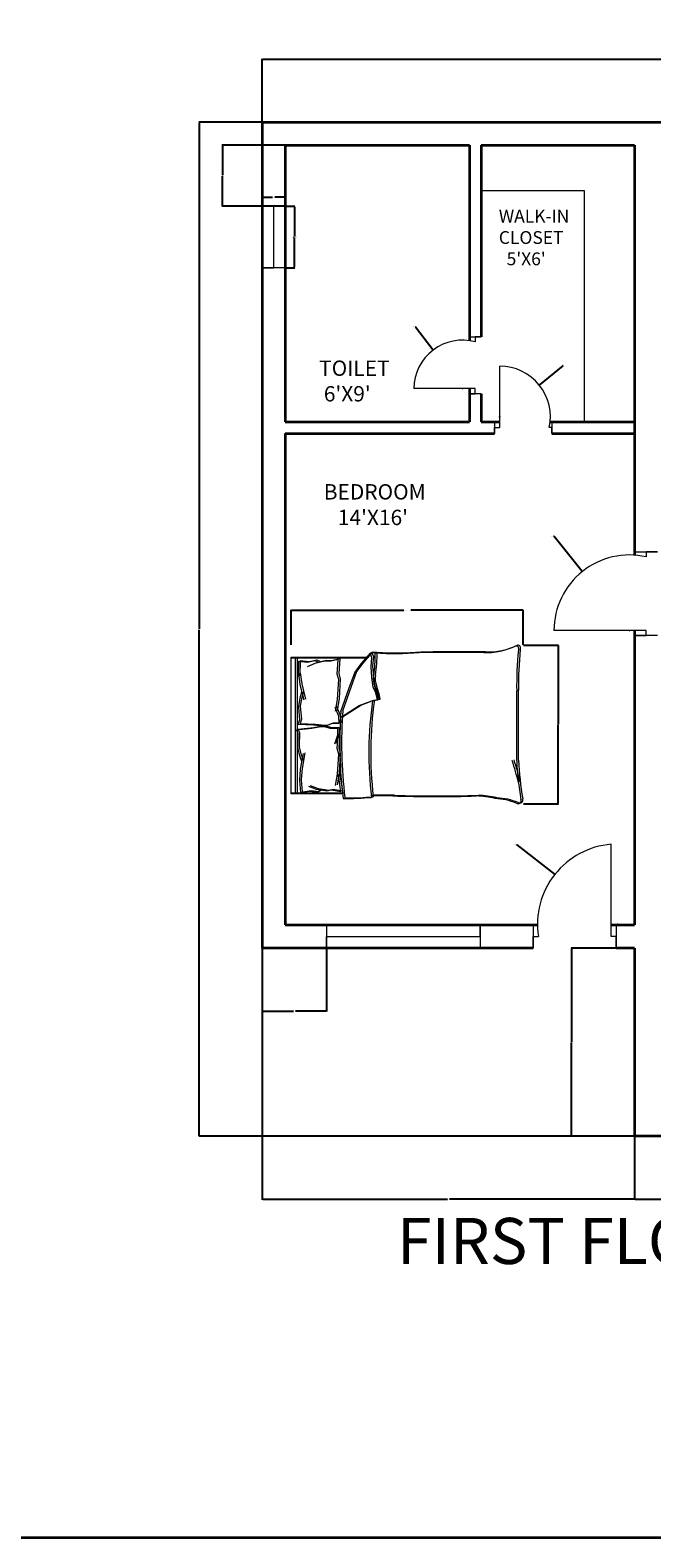
# Model space of a CAD drawing. Units: inches. Extents: x 2067 to 3463, y 1605 to 2723.
# Tile 8 of 10: x 2765 to 3008, y 1605 to 2194. Entities that reach past the tile are written whole.
import ezdxf

# ---------------------------------------------------------------- set-up
doc = ezdxf.new("R2010")
doc.units = ezdxf.units.IN
for name, color, linetype, lineweight in [('A-ANNO-DIMS', 2, 'Continuous', 18), ('A-ANNO-TEXT', 7, 'Continuous', 35), ('A-ANNO-TTLB', 7, 'Continuous', 35), ('A-AREA-IDEN', 7, 'Continuous', 18), ('A-DOOR', 3, 'Continuous', 18), ('A-FLOR-CASE', 8, 'Continuous', 18), ('A-FURN', 8, 'Continuous', 13), ('A-GLAZ', 4, 'Continuous', 18), ('A-WALL', 7, 'Continuous', 35)]:
    doc.layers.add(name, color=color, linetype=linetype, lineweight=lineweight)
doc.styles.get("Standard").update_dxf_attribs({"font": 'arial.ttf'})
doc.dimstyles.get("Standard").update_dxf_attribs({"dimtxt": 0.18, "dimasz": 0.18, "dimexe": 0.18, "dimexo": 0.0625, "dimgap": 0.09, "dimtad": 0, "dimtih": 1, "dimtoh": 1, "dimdec": 4, "dimzin": 0, "dimdsep": 46, "dimtxsty": 'Standard', "dimcen": 0.09, "dimadec": 0, "dimazin": 0, "dimtfac": 1, "dimtdec": 4, "dimtofl": 0, "dimtmove": 0, "dimatfit": 3, "dimfxl": 1, "dimtolj": 1, "dimtzin": 0, "dimarcsym": 0})

# ---------------------------------------------------------------- blocks, each defined once
blk = doc.blocks.new('BED-DOUBLE')
for p, q in [((3.86, 70.43), (3.86, 90.57)), ((3.86, 90.57), (57.01, 90.57)), ((3.86, 88.86), (57.01, 88.86)), ((4.12, 89.85), (4.12, 90.57)), ((4.12, 69.72), (4.12, 89.85)), ((27.29, 87.84), (28.89, 88.49)), ((28.89, 88.49), (29.54, 82.54)), ((57.01, 90.57), (57.01, 60.97)), ((57.01, 90.57), (57.26, 90.57)), ((57.26, 90.57), (57.26, 89.74)), ((57.26, 89.85), (57.26, 60.26)), ((4.12, 88.15), (57.26, 88.15)), ((4.33, 86.88), (4.97, 83.34)), ((4.34, 86.85), (9.1, 87.22)), ((4.97, 83.34), (4.49, 80.45)), ((4.59, 86.14), (9.35, 86.51)), ((4.59, 86.17), (5.23, 82.63)), ((5.23, 82.63), (4.75, 79.74)), ((5.62, 80.61), (6.74, 83.66)), ((5.87, 79.9), (7, 82.95)), ((9.1, 87.22), (9.21, 87.2)), ((9.21, 87.2), (13.46, 86.88)), ((9.35, 86.51), (9.47, 86.49)), ((9.47, 86.49), (13.72, 86.17)), ((13.46, 86.88), (19.57, 85.75)), ((13.72, 86.17), (19.83, 85.04)), ((16.52, 86.4), (18.77, 87.2)), ((16.77, 85.68), (19.02, 86.49)), ((18.77, 87.2), (21.98, 88)), ((19.02, 86.49), (22.24, 87.29)), ((21.98, 88), (22.34, 88)), ((22.24, 87.29), (22.6, 87.29)), ((22.34, 88), (27.29, 87.84)), ((22.6, 87.29), (27.54, 87.13)), ((27.54, 87.13), (29.15, 87.77)), ((29.15, 87.77), (29.79, 81.83)), ((29.54, 82.54), (30.18, 79)), ((31.11, 87.79), (30.84, 81.82)), ((31.36, 87.08), (31.09, 81.11)), ((32.76, 87.25), (31.11, 87.79)), ((33.01, 86.54), (31.36, 87.08)), ((37.68, 87.72), (32.76, 87.25)), ((37.93, 87.01), (33.01, 86.54)), ((38.04, 87.74), (37.68, 87.72)), ((38.29, 87.03), (37.93, 87.01)), ((41.29, 87.14), (38.04, 87.74)), ((41.55, 86.43), (38.29, 87.03)), ((46.61, 87.15), (40.58, 85.65)), ((46.86, 86.44), (40.84, 84.94)), ((43.59, 86.48), (41.29, 87.14)), ((43.85, 85.77), (41.55, 86.43)), ((50.83, 87.74), (46.61, 87.15)), ((51.09, 87.03), (46.86, 86.44)), ((55.73, 87.72), (49.72, 87.83)), ((49.72, 87.83), (50.83, 87.74)), ((55.98, 87.01), (49.97, 87.12)), ((49.97, 87.12), (51.09, 87.03)), ((54.83, 81.38), (53.52, 84.36)), ((55.09, 80.67), (53.77, 83.65)), ((55.73, 87.72), (55.3, 84.15)), ((55.3, 84.15), (55.97, 81.29)), ((55.98, 87.01), (55.56, 83.44)), ((55.56, 83.44), (56.22, 80.58)), ((4.49, 80.45), (5.13, 79.32)), ((4.75, 79.74), (5.39, 78.61)), ((4.97, 76.59), (5.62, 80.61)), ((5.3, 74.82), (4.97, 76.59)), ((5.23, 75.88), (5.87, 79.9)), ((30.18, 77.55), (29.54, 75.46)), ((29.79, 81.83), (30.43, 78.29)), ((30.43, 76.84), (29.79, 74.75)), ((30.18, 79), (30.18, 77.55)), ((30.84, 81.82), (30.42, 78.25)), ((30.42, 78.25), (30.51, 76.8)), ((30.43, 78.29), (30.43, 76.84)), ((30.51, 76.8), (31.28, 74.76)), ((31.09, 81.11), (30.67, 77.54)), ((30.67, 77.54), (30.76, 76.09)), ((55.73, 77.41), (54.83, 81.38)), ((55.98, 76.7), (55.09, 80.67)), ((55.97, 81.29), (55.39, 80.13)), ((55.51, 75.63), (55.73, 77.41)), ((56.22, 80.58), (55.65, 79.42)), ((55.77, 74.92), (55.98, 76.7)), ((4.65, 71.28), (5.3, 74.82)), ((10.32, 72.09), (4.65, 71.28)), ((4.91, 70.57), (5.55, 74.11)), ((10.57, 71.37), (4.91, 70.57)), ((5.55, 74.11), (5.23, 75.88)), ((7.1, 73.19), (11.58, 72.44)), ((7.35, 72.48), (11.83, 71.73)), ((11.58, 72.44), (10.32, 72.09)), ((11.83, 71.73), (10.57, 71.37)), ((11.58, 72.44), (19.38, 71.97)), ((11.83, 71.73), (19.63, 71.25)), ((19.38, 71.97), (21.56, 72.58)), ((19.63, 71.25), (21.81, 71.87)), ((21.56, 72.58), (27.26, 72.14)), ((21.81, 71.87), (27.52, 71.43)), ((26.8, 72.48), (23.31, 73.69)), ((27.06, 71.77), (23.56, 72.98)), ((29.54, 72.48), (26.8, 72.48)), ((29.79, 71.77), (27.06, 71.77)), ((29.54, 75.46), (29.54, 72.48)), ((29.79, 74.75), (29.79, 71.77)), ((30.76, 76.09), (31.54, 74.05)), ((31.28, 74.76), (31.47, 71.78)), ((31.47, 71.78), (34.19, 71.95)), ((31.54, 74.05), (31.72, 71.07)), ((31.72, 71.07), (34.45, 71.24)), ((33.65, 71.23), (38.31, 64.01)), ((34.19, 71.95), (37.61, 73.38)), ((34.45, 71.24), (37.86, 72.67)), ((45.2, 67.97), (35.92, 71.23)), ((36.21, 73.19), (40.7, 72.44)), ((36.47, 72.48), (40.95, 71.73)), ((40.7, 72.44), (48.49, 71.97)), ((40.95, 71.73), (48.74, 71.25)), ((48.49, 71.97), (50.67, 72.58)), ((48.74, 71.25), (50.92, 71.87)), ((50.67, 72.58), (56.38, 72.14)), ((50.92, 71.87), (56.63, 71.43)), ((56.38, 72.14), (55.51, 75.63)), ((56.63, 71.43), (55.77, 74.92)), ((33.9, 70.52), (38.56, 63.3)), ((45.45, 67.26), (36.18, 70.52)), ((51.4, 65.74), (45.2, 67.97)), ((51.65, 65.02), (45.45, 67.26)), ((54.67, 63.33), (51.4, 65.74)), ((54.92, 62.61), (51.65, 65.02)), ((38.31, 64.01), (40.2, 59.02)), ((38.56, 63.3), (40.46, 58.31)), ((40.2, 59.02), (40.55, 56.79)), ((45.54, 58.51), (49.33, 59.02)), ((49.33, 59.02), (53.64, 59.37)), ((53.64, 59.37), (57.08, 59.02)), ((58.79, 59.71), (54.67, 63.33)), ((59.04, 59), (54.92, 62.61)), ((57.08, 59.02), (58.79, 59.71)), ((57.33, 58.31), (59.04, 59)), ((58.88, 57.77), (58.79, 59.71, 4.3)), ((59.13, 57.06), (59.04, 59, 4.3)), ((40.46, 58.31), (40.8, 56.07)), ((40.55, 56.79), (43.3, 57.47)), ((40.8, 56.07), (43.56, 56.76)), ((43.3, 57.47), (45.54, 58.51)), ((43.56, 56.76), (45.8, 57.8)), ((45.8, 57.8), (49.58, 58.31)), ((49.58, 58.31), (53.89, 58.66)), ((53.89, 58.66), (57.33, 58.31)), ((16.75, 2.44), (44.12, 2.44)), ((17, 1.73), (44.38, 1.73))]:
    blk.add_line(p, q)
for centre, radius, start, end in [((23.75, -111.88), 183.45, 86.08655, 96.78213), ((24.01, -112.59), 183.45, 86.08655, 96.78213), ((94.7, 68.22), 92.64, 178.72178, 185.60397), ((94.95, 67.51), 92.64, 178.72178, 185.60397), ((19.74, -83.26), 143.47, 81.78449, 96.90062), ((20, -83.97), 143.47, 81.78449, 96.90062), ((-186.05, 55.9), 189.16, 358.4762, 1.00819), ((-185.79, 55.19), 189.16, 358.4762, 1.00819), ((40.74, 56.72), 0.205, 160.24637, 271.13765), ((34.64, 88.92), 32.98, 280.66171, 289.88058), ((40.99, 56.01), 0.205, 160.24637, 271.13765), ((34.9, 88.21), 32.98, 280.66171, 289.88058), ((48.64, 51.57), 6.92, 78.6608, 113.73842), ((48.9, 50.86), 6.92, 78.6608, 113.73842), ((57.08, 97.97), 40.24, 259.87628, 272.56571), ((57.33, 97.26), 40.24, 259.87628, 272.56571), ((202.68, 50.18), 144, 176.97912, 183.83645), ((202.94, 49.47), 144, 176.97912, 183.83645), ((539.13, 34.28), 536.33, 178.22771, 181.71854), ((539.38, 33.57), 536.33, 178.22771, 181.71854), ((-5013.77, 15.15), 5072.83, 0.00217, 0.28689), ((-5013.52, 14.44), 5072.83, 0.00217, 0.28689), ((-29.91, 18.82), 32.95, 346.06484, 358.91125), ((-29.66, 18.11), 32.95, 346.06484, 358.91125), ((84.69, 14.21), 25.65, 177.47136, 206.46809), ((84.94, 13.5), 25.65, 177.47136, 206.46809), ((-24.09, 12.42), 26.2, 337.97508, 356.652), ((-23.83, 11.71), 26.2, 337.97508, 356.652), ((1.21, 1.92), 1.21, 146.17358, 293.47814), ((1.46, 1.21), 1.21, 146.17358, 293.47814), ((23.83, -132.77), 135.4, 92.99578, 99.40907), ((24.08, -133.48), 135.4, 92.99578, 99.40907), ((-19.15, 116.93), 118.38, 283.38322, 287.70533), ((-18.9, 116.22), 118.38, 283.38322, 287.70533), ((45.76, -145.49), 147.94, 84.4998, 90.63509), ((46.02, -146.2), 147.94, 84.4998, 90.63509), ((60.5, 2.86), 1.23, 242.65876, 356.02002), ((60.76, 2.15), 1.23, 242.65876, 356.02002)]:
    blk.add_arc(centre, radius, start, end)
blk = doc.blocks.new('WIN-PLAN-24-ALIGNED')
for p, q in [((0, 0), (0, 9)), ((0, 9), (0, 4.5)), ((24, 4.5), (24, 9)), ((24, 9), (24, 0)), ((0, 4.5), (24, 4.5))]:
    blk.add_line(p, q)
blk = doc.blocks.new('WIN-PLAN-60-OFFSET')
for p, q in [((0, 9), (0, 0)), ((60, 4.5), (60, 9)), ((60, 9), (60, 0)), ((0, 0), (0, 4.5)), ((0, 4.5), (60, 4.5))]:
    blk.add_line(p, q)
blk = doc.blocks.new('*D10')
at = {"layer": 'A-ANNO-DIMS', "color": 0, "lineweight": -2, "transparency": 16777216}
for p, q in [((2867.3, 1954.12), (2867.3, 1967.84)), ((2867.48, 1967.66), (2911.27, 1967.66)), ((2957.8, 1967.66), (2914.01, 1967.66)), ((2957.98, 1954.12), (2957.98, 1967.84))]:
    blk.add_line(p, q, dxfattribs=at)
at = {"layer": 'A-ANNO-DIMS', "color": 0, "transparency": 16777216}
for points in [[(2867.48, 1967.69), (2867.48, 1967.63), (2867.3, 1967.66)], [(2957.8, 1967.69), (2957.8, 1967.63), (2957.98, 1967.66)]]:
    blk.add_solid(points, dxfattribs=at)
at = {"layer": 'Defpoints', "color": 0, "transparency": 16777216}
for p in [(2867.3, 1967.66), (2867.3, 1954.06), (2957.98, 1954.06)]:
    blk.add_point(p, dxfattribs=at)
at = {"layer": 'A-ANNO-DIMS', "color": 0, "transparency": 16777216, "insert": (2912.64, 1967.66), "char_height": 0.18, "attachment_point": 5}
blk.add_mtext('\\A1;DOUBLE BED 91 TYP.', dxfattribs=at)
blk = doc.blocks.new('*D11')
at = {"layer": 'A-ANNO-DIMS', "color": 0, "lineweight": -2, "transparency": 16777216}
for p, q in [((2958.04, 1954.06), (2971.76, 1954.06)), ((2971.58, 1953.88), (2971.58, 1923.2)), ((2971.58, 1892.16), (2971.58, 1922.84)), ((2958.04, 1891.98), (2971.76, 1891.98))]:
    blk.add_line(p, q, dxfattribs=at)
at = {"layer": 'A-ANNO-DIMS', "color": 0, "transparency": 16777216}
for points in [[(2971.55, 1953.88), (2971.61, 1953.88), (2971.58, 1954.06)], [(2971.55, 1892.16), (2971.61, 1892.16), (2971.58, 1891.98)]]:
    blk.add_solid(points, dxfattribs=at)
at = {"layer": 'Defpoints', "color": 0, "transparency": 16777216}
for p in [(2957.98, 1954.06), (2971.58, 1954.06), (2957.98, 1891.98)]:
    blk.add_point(p, dxfattribs=at)
at = {"layer": 'A-ANNO-DIMS', "color": 0, "transparency": 16777216, "insert": (2971.58, 1923.02), "char_height": 0.18, "attachment_point": 5}
blk.add_mtext('\\A1;62 TYP.', dxfattribs=at)
blk = doc.blocks.new('*D20')
at = {"layer": 'A-ANNO-DIMS', "color": 0, "lineweight": -2, "transparency": 16777216}
for p, q in [((2865.06, 2125.4), (2868.78, 2125.4)), ((2868.6, 2125.22), (2868.6, 2113.58)), ((2868.6, 2101.58), (2868.6, 2113.22)), ((2865.06, 2101.4), (2868.78, 2101.4))]:
    blk.add_line(p, q, dxfattribs=at)
at = {"layer": 'A-ANNO-DIMS', "color": 0, "transparency": 16777216}
for points in [[(2868.57, 2125.22), (2868.63, 2125.22), (2868.6, 2125.4)], [(2868.57, 2101.58), (2868.63, 2101.58), (2868.6, 2101.4)]]:
    blk.add_solid(points, dxfattribs=at)
at = {"layer": 'Defpoints', "color": 0, "transparency": 16777216}
for p in [(2865, 2125.4), (2868.6, 2125.4), (2865, 2101.4)]:
    blk.add_point(p, dxfattribs=at)
at = {"layer": 'A-ANNO-DIMS', "color": 0, "transparency": 16777216, "insert": (2868.6, 2113.4), "char_height": 0.18, "attachment_point": 5}
blk.add_mtext('\\A1;WINDOW 24 TYP.', dxfattribs=at)
blk = doc.blocks.new('*D21')
at = {"layer": 'A-ANNO-DIMS', "color": 0, "lineweight": -2, "transparency": 16777216}
for p, q in [((2856, 2125.46), (2856, 2129.18)), ((2856.18, 2129), (2860.04, 2129)), ((2864.82, 2129), (2860.96, 2129)), ((2865, 2125.46), (2865, 2129.18))]:
    blk.add_line(p, q, dxfattribs=at)
at = {"layer": 'A-ANNO-DIMS', "color": 0, "transparency": 16777216}
for points in [[(2856.18, 2129.03), (2856.18, 2128.97), (2856, 2129)], [(2864.82, 2129.03), (2864.82, 2128.97), (2865, 2129)]]:
    blk.add_solid(points, dxfattribs=at)
at = {"layer": 'Defpoints', "color": 0, "transparency": 16777216}
for p in [(2856, 2129), (2856, 2125.4), (2865, 2125.4)]:
    blk.add_point(p, dxfattribs=at)
at = {"layer": 'A-ANNO-DIMS', "color": 0, "transparency": 16777216, "insert": (2860.5, 2129), "char_height": 0.18, "attachment_point": 5}
blk.add_mtext('\\A1;9 TYP.', dxfattribs=at)
blk = doc.blocks.new('*D50')
at = {"layer": 'A-ANNO-DIMS', "color": 0, "lineweight": -2, "transparency": 16777216}
for p, q in [((2856, 2158.29), (2856, 2183.01)), ((2856.18, 2182.83), (3053.71, 2182.83)), ((3251.82, 2182.83), (3054.29, 2182.83)), ((3252, 2158.29), (3252, 2183.01))]:
    blk.add_line(p, q, dxfattribs=at)
at = {"layer": 'A-ANNO-DIMS', "color": 0, "transparency": 16777216}
for points in [[(2856.18, 2182.86), (2856.18, 2182.8), (2856, 2182.83)], [(3251.82, 2182.86), (3251.82, 2182.8), (3252, 2182.83)]]:
    blk.add_solid(points, dxfattribs=at)
at = {"layer": 'Defpoints', "color": 0, "transparency": 16777216}
for p in [(3252, 2182.83), (2856, 2158.23), (3252, 2158.23)]:
    blk.add_point(p, dxfattribs=at)
at = {"layer": 'A-ANNO-DIMS', "color": 0, "transparency": 16777216, "insert": (3054, 2182.83), "char_height": 0.18, "attachment_point": 5}
blk.add_mtext('\\A1;396', dxfattribs=at)
blk = doc.blocks.new('*D51')
at = {"layer": 'A-ANNO-DIMS', "color": 0, "lineweight": -2, "transparency": 16777216}
for p, q in [((2855.94, 2158.23), (2831.22, 2158.23)), ((2831.4, 2158.05), (2831.4, 1960.41)), ((2831.4, 1762.41), (2831.4, 1960.05)), ((3001.44, 1762.23), (2831.22, 1762.23))]:
    blk.add_line(p, q, dxfattribs=at)
at = {"layer": 'A-ANNO-DIMS', "color": 0, "transparency": 16777216}
for points in [[(2831.37, 2158.05), (2831.43, 2158.05), (2831.4, 2158.23)], [(2831.37, 1762.41), (2831.43, 1762.41), (2831.4, 1762.23)]]:
    blk.add_solid(points, dxfattribs=at)
at = {"layer": 'Defpoints', "color": 0, "transparency": 16777216}
for p in [(2856, 2158.23), (2831.4, 1762.23), (3001.5, 1762.23)]:
    blk.add_point(p, dxfattribs=at)
at = {"layer": 'A-ANNO-DIMS', "color": 0, "transparency": 16777216, "insert": (2831.4, 1960.23), "char_height": 0.18, "attachment_point": 5}
blk.add_mtext('\\A1;396', dxfattribs=at)
blk = doc.blocks.new('*D52')
at = {"layer": 'A-ANNO-DIMS', "color": 0, "lineweight": -2, "transparency": 16777216}
for p, q in [((2856, 1835.67), (2856, 1737.45)), ((3001.5, 1835.67), (3001.5, 1737.45)), ((2856.18, 1737.63), (2928.36, 1737.63)), ((3001.32, 1737.63), (2929.14, 1737.63))]:
    blk.add_line(p, q, dxfattribs=at)
at = {"layer": 'A-ANNO-DIMS', "color": 0, "transparency": 16777216}
for points in [[(2856.18, 1737.66), (2856.18, 1737.6), (2856, 1737.63)], [(3001.32, 1737.66), (3001.32, 1737.6), (3001.5, 1737.63)]]:
    blk.add_solid(points, dxfattribs=at)
at = {"layer": 'Defpoints', "color": 0, "transparency": 16777216}
for p in [(2856, 1835.73), (3001.5, 1835.73), (3001.5, 1737.63)]:
    blk.add_point(p, dxfattribs=at)
at = {"layer": 'A-ANNO-DIMS', "color": 0, "transparency": 16777216, "insert": (2928.75, 1737.63), "char_height": 0.18, "attachment_point": 5}
blk.add_mtext('\\A1;145.5', dxfattribs=at)
blk = doc.blocks.new('*D53')
at = {"layer": 'A-ANNO-DIMS', "color": 0, "lineweight": -2, "transparency": 16777216}
for p, q in [((3001.5, 1762.17), (3001.5, 1737.45)), ((3031.71, 1762.17), (3031.71, 1737.45)), ((3001.68, 1737.63), (3016.14, 1737.63)), ((3031.53, 1737.63), (3017.07, 1737.63))]:
    blk.add_line(p, q, dxfattribs=at)
at = {"layer": 'A-ANNO-DIMS', "color": 0, "transparency": 16777216}
for points in [[(3001.68, 1737.66), (3001.68, 1737.6), (3001.5, 1737.63)], [(3031.53, 1737.66), (3031.53, 1737.6), (3031.71, 1737.63)]]:
    blk.add_solid(points, dxfattribs=at)
at = {"layer": 'Defpoints', "color": 0, "transparency": 16777216}
for p in [(3001.5, 1762.23), (3031.71, 1762.23), (3031.71, 1737.63)]:
    blk.add_point(p, dxfattribs=at)
at = {"layer": 'A-ANNO-DIMS', "color": 0, "transparency": 16777216, "insert": (3016.61, 1737.63), "char_height": 0.18, "attachment_point": 5}
blk.add_mtext('\\A1;30.215', dxfattribs=at)
blk = doc.blocks.new('*D56')
at = {"layer": 'A-ANNO-DIMS', "color": 0, "lineweight": -2, "transparency": 16777216}
for p, q in [((3001.44, 1835.73), (2976.72, 1835.73)), ((2976.9, 1835.55), (2976.9, 1799.16)), ((2976.9, 1762.41), (2976.9, 1798.8)), ((3001.44, 1762.23), (2976.72, 1762.23))]:
    blk.add_line(p, q, dxfattribs=at)
at = {"layer": 'A-ANNO-DIMS', "color": 0, "transparency": 16777216}
for points in [[(2976.87, 1835.55), (2976.93, 1835.55), (2976.9, 1835.73)], [(2976.87, 1762.41), (2976.93, 1762.41), (2976.9, 1762.23)]]:
    blk.add_solid(points, dxfattribs=at)
at = {"layer": 'Defpoints', "color": 0, "transparency": 16777216}
for p in [(2976.9, 1835.73), (3001.5, 1835.73), (3001.5, 1762.23)]:
    blk.add_point(p, dxfattribs=at)
at = {"layer": 'A-ANNO-DIMS', "color": 0, "transparency": 16777216, "insert": (2976.9, 1798.98), "char_height": 0.18, "attachment_point": 5}
blk.add_mtext('\\A1;73.5', dxfattribs=at)
blk = doc.blocks.new('*D61')
at = {"layer": 'A-ANNO-DIMS', "color": 0, "lineweight": -2, "transparency": 16777216}
for p, q in [((2856, 1835.67), (2856, 1810.95)), ((2881.11, 1835.67), (2881.11, 1810.95)), ((2856.18, 1811.13), (2868.18, 1811.13)), ((2880.93, 1811.13), (2868.93, 1811.13))]:
    blk.add_line(p, q, dxfattribs=at)
at = {"layer": 'A-ANNO-DIMS', "color": 0, "transparency": 16777216}
for points in [[(2856.18, 1811.16), (2856.18, 1811.1), (2856, 1811.13)], [(2880.93, 1811.16), (2880.93, 1811.1), (2881.11, 1811.13)]]:
    blk.add_solid(points, dxfattribs=at)
at = {"layer": 'Defpoints', "color": 0, "transparency": 16777216}
for p in [(2856, 1835.73), (2881.11, 1835.73), (2856, 1811.13)]:
    blk.add_point(p, dxfattribs=at)
at = {"layer": 'A-ANNO-DIMS', "color": 0, "transparency": 16777216, "insert": (2868.56, 1811.13), "char_height": 0.18, "attachment_point": 5}
blk.add_mtext('\\A1;25.11', dxfattribs=at)
blk = doc.blocks.new('*D62')
at = {"layer": 'A-ANNO-DIMS', "color": 0, "lineweight": -2, "transparency": 16777216}
for p, q in [((2864.94, 2149.23), (2840.22, 2149.23)), ((2840.4, 2149.05), (2840.4, 2137.5)), ((2840.4, 2125.58), (2840.4, 2137.13)), ((2864.94, 2125.4), (2840.22, 2125.4))]:
    blk.add_line(p, q, dxfattribs=at)
at = {"layer": 'A-ANNO-DIMS', "color": 0, "transparency": 16777216}
for points in [[(2840.37, 2149.05), (2840.43, 2149.05), (2840.4, 2149.23)], [(2840.37, 2125.58), (2840.43, 2125.58), (2840.4, 2125.4)]]:
    blk.add_solid(points, dxfattribs=at)
at = {"layer": 'Defpoints', "color": 0, "transparency": 16777216}
for p in [(2840.4, 2149.23), (2865, 2149.23), (2865, 2125.4)]:
    blk.add_point(p, dxfattribs=at)
at = {"layer": 'A-ANNO-DIMS', "color": 0, "transparency": 16777216, "insert": (2840.4, 2137.32), "char_height": 0.18, "attachment_point": 5}
blk.add_mtext('\\A1;23.83', dxfattribs=at)
blk = doc.blocks.new('*D108')
at = {"layer": 'A-ANNO-DIMS', "color": 0, "lineweight": -2, "transparency": 16777216}
for p, q in [((2955.36, 1876.07), (2955.54, 1876.07)), ((2955.54, 1876.07), (2970.14, 1864.54)), ((2994.76, 1845.03), (2994.94, 1845.03)), ((2994.85, 1844.94), (2994.85, 1845.12))]:
    blk.add_line(p, q, dxfattribs=at)
at = {"layer": 'A-ANNO-DIMS', "color": 0, "transparency": 16777216}
blk.add_solid([(2970.16, 1864.57), (2970.12, 1864.52), (2970.28, 1864.43)], dxfattribs=at)
at = {"layer": 'Defpoints', "color": 0, "transparency": 16777216}
for p in [(2970.28, 1864.43), (2994.85, 1845.03)]:
    blk.add_point(p, dxfattribs=at)
at = {"layer": 'A-ANNO-DIMS', "color": 0, "transparency": 16777216, "insert": (2954.81, 1876.07), "char_height": 0.18, "attachment_point": 5}
blk.add_mtext('\\A1;R31.305', dxfattribs=at)
blk = doc.blocks.new('*D110')
at = {"layer": 'A-ANNO-DIMS', "color": 0, "lineweight": -2, "transparency": 16777216}
for p, q in [((2969.87, 1996.61), (2970.05, 1996.61)), ((2970.05, 1996.61), (2980.97, 1982.93)), ((2999.39, 1959.75), (2999.57, 1959.75)), ((2999.48, 1959.66), (2999.48, 1959.84))]:
    blk.add_line(p, q, dxfattribs=at)
at = {"layer": 'A-ANNO-DIMS', "color": 0, "transparency": 16777216}
blk.add_solid([(2980.99, 1982.95), (2980.95, 1982.91), (2981.08, 1982.79)], dxfattribs=at)
at = {"layer": 'Defpoints', "color": 0, "transparency": 16777216}
for p in [(2981.08, 1982.79), (2999.48, 1959.75)]:
    blk.add_point(p, dxfattribs=at)
at = {"layer": 'A-ANNO-DIMS', "color": 0, "transparency": 16777216, "insert": (2969.32, 1996.61), "char_height": 0.18, "attachment_point": 5}
blk.add_mtext('\\A1;R29.477', dxfattribs=at)
blk = doc.blocks.new('*D112')
at = {"layer": 'A-ANNO-DIMS', "color": 0, "lineweight": -2, "transparency": 16777216}
for p, q in [((2973.46, 2063.05), (2964.36, 2055.72)), ((2973.64, 2063.05), (2973.46, 2063.05)), ((2948.72, 2043.2), (2948.9, 2043.2)), ((2948.81, 2043.11), (2948.81, 2043.29))]:
    blk.add_line(p, q, dxfattribs=at)
at = {"layer": 'A-ANNO-DIMS', "color": 0, "transparency": 16777216}
blk.add_solid([(2964.34, 2055.74), (2964.38, 2055.7), (2964.22, 2055.61)], dxfattribs=at)
at = {"layer": 'Defpoints', "color": 0, "transparency": 16777216}
for p in [(2964.22, 2055.61), (2948.81, 2043.2)]:
    blk.add_point(p, dxfattribs=at)
at = {"layer": 'A-ANNO-DIMS', "color": 0, "transparency": 16777216, "insert": (2974.19, 2063.05), "char_height": 0.18, "attachment_point": 5}
blk.add_mtext('\\A1;R19.785', dxfattribs=at)
blk = doc.blocks.new('*D113')
at = {"layer": 'A-ANNO-DIMS', "color": 0, "lineweight": -2, "transparency": 16777216}
for p, q in [((2915.69, 2078.31), (2915.87, 2078.31)), ((2915.87, 2078.31), (2922.62, 2069.41)), ((2934.07, 2054.21), (2934.25, 2054.21)), ((2934.16, 2054.12), (2934.16, 2054.3))]:
    blk.add_line(p, q, dxfattribs=at)
at = {"layer": 'A-ANNO-DIMS', "color": 0, "transparency": 16777216}
blk.add_solid([(2922.64, 2069.43), (2922.6, 2069.39), (2922.73, 2069.27)], dxfattribs=at)
at = {"layer": 'Defpoints', "color": 0, "transparency": 16777216}
for p in [(2922.73, 2069.27), (2934.16, 2054.21)]:
    blk.add_point(p, dxfattribs=at)
at = {"layer": 'A-ANNO-DIMS', "color": 0, "transparency": 16777216, "insert": (2915.23, 2078.31), "char_height": 0.18, "attachment_point": 5}
blk.add_mtext('\\A1;R18.91', dxfattribs=at)

msp = doc.modelspace()

# ---------------------------------------------------------------- linework, layer by layer
at = {"layer": 'A-ANNO-TTLB'}
msp.add_lwpolyline([(2067.2624, 2722.6321), (3463.3053, 2722.6321), (3463.3053, 1605.3918), (2067.2624, 1605.3918)], close=True, dxfattribs=at)
at = {"layer": 'A-DOOR'}
for p, q in [((2936.9994, 2074.416), (2941.4994, 2074.416)), ((2941.4994, 2074.416), (2939.2494, 2074.416)), ((2939.2494, 2074.416), (2939.2494, 2072.416)), ((2948.8099, 2038.9809), (2948.8099, 2062.9809)), ((2939.2494, 2054.2055), (2915.2494, 2054.2055)), ((2941.4994, 2052.2055), (2936.9994, 2052.2055)), ((2936.9994, 2052.2055), (2939.2494, 2052.2055)), ((2939.2494, 2052.2055), (2939.2494, 2054.2055)), ((2939.2494, 2052.2055), (2939.2494, 2052.2055)), ((2946.8099, 2041.2309), (2946.8099, 2036.7309)), ((2946.8099, 2036.7309), (2946.8099, 2038.9809)), ((2946.8099, 2038.9809), (2948.8099, 2038.9809)), ((2969.1412, 2038.9809), (2968.1412, 2038.9809)), ((2969.1412, 2041.2309), (2969.1412, 2036.7309)), ((2969.1412, 2036.7309), (2969.1412, 2038.9809)), ((3001.4994, 1990.4993), (3010.4994, 1990.4993)), ((3010.4994, 1990.4993), (3005.9994, 1990.4993)), ((3005.9994, 1990.4993), (3005.9994, 1988.4993)), ((3005.9994, 1959.7531), (2969.9994, 1959.7531)), ((3010.4994, 1957.7531), (3001.4994, 1957.7531)), ((3001.4994, 1957.7531), (3005.9994, 1957.7531)), ((3005.9994, 1957.7531), (3005.9994, 1959.7531)), ((2992.3492, 1840.2309), (2992.3492, 1876.2309)), ((2961.9105, 1844.7309), (2961.9105, 1835.7309)), ((2994.3492, 1844.7309), (2994.3492, 1835.7309)), ((2961.9105, 1835.7309), (2961.9105, 1840.2309)), ((2961.9105, 1840.2309), (2963.9105, 1840.2309)), ((2994.3492, 1840.2309), (2992.3492, 1840.2309)), ((2994.3492, 1835.7309), (2994.3492, 1840.2309))]:
    msp.add_line(p, q, dxfattribs=at)
for centre, radius, start, end in [((2934.1583, 2054.2055), 18.9088, 74.3804694, 180), ((2948.8099, 2043.1954), 19.7854, 347.7009247, 90), ((2999.4764, 1959.7531), 29.477, 77.2151522, 180), ((2994.8457, 1845.026), 31.3046, 94.5741512, 188.8110553)]:
    msp.add_arc(centre, radius, start, end, dxfattribs=at)
at = {"layer": 'A-FLOR-CASE'}
for p, q in [((2941.4994, 2131.5966), (2981.8583, 2131.5966)), ((2981.8583, 2131.5966), (2981.8583, 2041.2309))]:
    msp.add_line(p, q, dxfattribs=at)
at = {"layer": 'A-GLAZ'}
for p, q in [((2860.4994, 2125.4017), (2860.4994, 2125.4017)), ((2855.9994, 2101.4017), (2855.9994, 2101.4017))]:
    msp.add_line(p, q, dxfattribs=at)
at = {"layer": 'A-WALL'}
for p, q in [((2855.9994, 2158.2309), (3251.9994, 2158.2309)), ((2855.9994, 2158.2309), (2855.9994, 1835.7309)), ((2864.9994, 2149.2309), (2936.9994, 2149.2309)), ((2864.9994, 2149.2309), (2864.9994, 2041.2309)), ((2936.9994, 2149.2309), (2936.9994, 2072.8996)), ((2941.4994, 2149.2309), (2941.4994, 2074.416)), ((2941.4994, 2149.2309), (3001.4994, 2149.2309)), ((3001.4994, 2149.2309), (3001.4994, 1989.1606)), ((2936.9994, 2054.2055), (2936.9994, 2041.2309)), ((2941.4994, 2052.2055), (2941.4994, 2041.2309)), ((2864.9994, 2041.2309), (2933.5851, 2041.2309)), ((2931.5851, 2041.2309), (2936.9994, 2041.2309)), ((2941.4994, 2041.2309), (2948.8099, 2041.2309)), ((2968.4975, 2041.2309), (3001.4994, 2041.2309)), ((2864.9994, 2036.7309), (2933.5851, 2036.7309)), ((2864.9994, 2036.7309), (2864.9994, 1844.7309)), ((2864.9994, 2036.7309), (2864.9994, 1844.7309)), ((2933.5851, 2036.7309), (2936.9994, 2036.7309)), ((2936.9994, 2036.7309), (2946.8099, 2036.7309)), ((2969.1412, 2036.7309), (3001.4994, 2036.7309)), ((3001.4994, 1959.7531), (3001.4994, 1844.7309)), ((2864.9994, 1844.7309), (2963.5425, 1844.7309)), ((2992.3492, 1844.7309), (3001.4994, 1844.7309)), ((2961.9105, 1835.7309), (2855.9994, 1835.7309)), ((3001.4994, 1835.7309), (2994.3492, 1835.7309)), ((3001.4994, 1835.7309), (3001.4994, 1762.2309)), ((3038.9994, 1762.2309), (3001.4994, 1762.2309))]:
    msp.add_line(p, q, dxfattribs=at)

# ---------------------------------------------------------------- block references
at = {"layer": 'A-FURN', "rotation": 89.99999999999991}
msp.add_blockref('BED-DOUBLE', (2957.8617, 1892.0743), dxfattribs=at)
at = {"layer": 'A-GLAZ', "rotation": 90.00000000000081}
msp.add_blockref('WIN-PLAN-24-ALIGNED', (2864.9993, 2101.4018), dxfattribs=at)
at = {"layer": 'A-GLAZ'}
msp.add_blockref('WIN-PLAN-60-OFFSET', (2881.111, 1835.731), dxfattribs=at)

# ---------------------------------------------------------------- texts
at = {"layer": 'A-ANNO-TEXT', "insert": (2908.6072, 1730.3295), "char_height": 18, "attachment_point": 1}
msp.add_mtext_dynamic_manual_height_columns('FIRST FLOOR PLAN', width=399.538466, gutter_width=12.5, heights=[0], dxfattribs=at)
at = {"layer": 'A-AREA-IDEN', "attachment_point": 1}
for s, width, insert, char_height in [("WALK-IN\\PCLOSET\\P  5'X6'", 34.584612, (2948.4374, 2124.0395), 5), ("TOILET\\P 6'X9'", 62.399063, (2878.2229, 2065.171), 6), ("BEDROOM\\P   14'X16'", 105.635915, (2880.0346, 2016.8895), 6)]:
    msp.add_mtext_dynamic_manual_height_columns(s, width=width, gutter_width=12.5, heights=[0], dxfattribs=dict(at, insert=insert, char_height=char_height))

# ---------------------------------------------------------------- dimensions: what is measured, and where the dimension line sits
at = {"layer": 'A-ANNO-DIMS'}
for base, p1, p2, override, picture, middle in [((3251.9994, 2182.8309), (2855.9994, 2158.2309), (3251.9994, 2158.2309), {"dimdec": 0, "dimlfac": 1, "dimrnd": 0, "dimzin": 0, "dimdsep": 46, "dimlunit": 2}, '*D50', (3053.9994, 2182.8309)), ((3001.4994, 1737.6309), (2855.9994, 1835.7309), (3001.4994, 1835.7309), {"dimdec": 1, "dimlfac": 1, "dimrnd": 0, "dimzin": 0, "dimdsep": 46, "dimlunit": 2}, '*D52', (2928.7494, 1737.6309)), ((3031.7142, 1737.6309), (3001.4994, 1762.2309), (3031.7142, 1762.2309), {"dimdec": 3, "dimlfac": 1, "dimrnd": 0, "dimzin": 0, "dimdsep": 46, "dimlunit": 2}, '*D53', (3016.6068, 1737.6309))]:
    dim = msp.add_linear_dim(base=base, p1=p1, p2=p2, dimstyle='Standard', override=override, dxfattribs=at)
    dim.commit()
    dim.dimension.update_dxf_attribs({"geometry": picture, "text_midpoint": middle})
for base, p1, p2, angle, override, picture, middle in [((2831.3994, 1762.2309), (2855.9994, 2158.2309), (3001.4994, 1762.2309), 90, {"dimdec": 0, "dimlfac": 1, "dimrnd": 0, "dimzin": 0, "dimdsep": 46, "dimlunit": 2}, '*D51', (2831.3994, 1960.2309)), ((2840.3994, 2149.2309), (2864.9994, 2125.4017), (2864.9994, 2149.2309), 90, {"dimdec": 2, "dimlfac": 1, "dimrnd": 0, "dimzin": 0, "dimdsep": 46, "dimlunit": 2}, '*D62', (2840.3994, 2137.3163)), ((2855.9994, 1811.1309), (2881.1112, 1835.7309), (2855.9994, 1835.7309), 180, {"dimdec": 2, "dimlfac": 1, "dimrnd": 0, "dimzin": 0, "dimdsep": 46, "dimlunit": 2}, '*D61', (2868.5553, 1811.1309)), ((2976.8994, 1835.7309), (3001.4994, 1762.2309), (3001.4994, 1835.7309), 90, {"dimdec": 1, "dimlfac": 1, "dimrnd": 0, "dimzin": 0, "dimdsep": 46, "dimlunit": 2}, '*D56', (2976.8994, 1798.9809))]:
    dim = msp.add_linear_dim(base=base, p1=p1, p2=p2, angle=angle, dimstyle='Standard', override=override, dxfattribs=at)
    dim.commit()
    dim.dimension.update_dxf_attribs({"geometry": picture, "text_midpoint": middle})
for base, p1, p2, angle, text, picture, middle in [((2855.9994, 2129.0017), (2864.9994, 2125.4017), (2855.9994, 2125.4017), 180, '<> TYP.', '*D21', (2860.4994, 2129.0017)), ((2868.5994, 2125.4017), (2864.9994, 2101.4017), (2864.9994, 2125.4017), 90, 'WINDOW <> TYP.', '*D20', (2868.5994, 2113.4017)), ((2867.2964, 1967.6582), (2957.9793, 1954.0558), (2867.2964, 1954.0558), 180, 'DOUBLE BED <> TYP.', '*D10', (2912.6378, 1967.6582)), ((2971.5817, 1954.0558), (2957.9793, 1891.9786), (2957.9793, 1954.0558), 90, '<> TYP.', '*D11', (2971.5817, 1923.0172))]:
    dim = msp.add_linear_dim(base=base, p1=p1, p2=p2, angle=angle, text=text, dimstyle='Standard', override={"dimdec": 0, "dimlfac": 1, "dimrnd": 0, "dimzin": 0, "dimdsep": 46, "dimlunit": 2}, dxfattribs=at)
    dim.commit()
    dim.dimension.update_dxf_attribs({"geometry": picture, "text_midpoint": middle})
for center, mpoint, override, picture, middle in [((2934.1583, 2054.2055), (2922.7289, 2069.2691), {"dimdec": 2, "dimlfac": 1, "dimrnd": 0, "dimzin": 0, "dimdsep": 46, "dimlunit": 2}, '*D113', (2915.2288, 2078.3073)), ((2948.8099, 2043.1954), (2964.2181, 2055.6071), {"dimdec": 3, "dimlfac": 1, "dimrnd": 0, "dimzin": 0, "dimdsep": 46, "dimlunit": 2}, '*D112', (2974.1935, 2063.0541)), ((2999.4764, 1959.7531), (2981.0833, 1982.7876), {"dimdec": 3, "dimlfac": 1, "dimrnd": 0, "dimzin": 0, "dimdsep": 46, "dimlunit": 2}, '*D110', (2969.3177, 1996.6083)), ((2994.8457, 1845.026), (2970.281, 1864.431), {"dimdec": 3, "dimlfac": 1, "dimrnd": 0, "dimzin": 0, "dimdsep": 46, "dimlunit": 2}, '*D108', (2954.8118, 1876.074))]:
    dim = msp.add_radius_dim(center=center, mpoint=mpoint, dimstyle='Standard', override=override, dxfattribs=at)
    dim.commit()
    dim.dimension.update_dxf_attribs({"geometry": picture, "text_midpoint": middle, "dimtype": 164})

doc.saveas('drawing.dxf')
